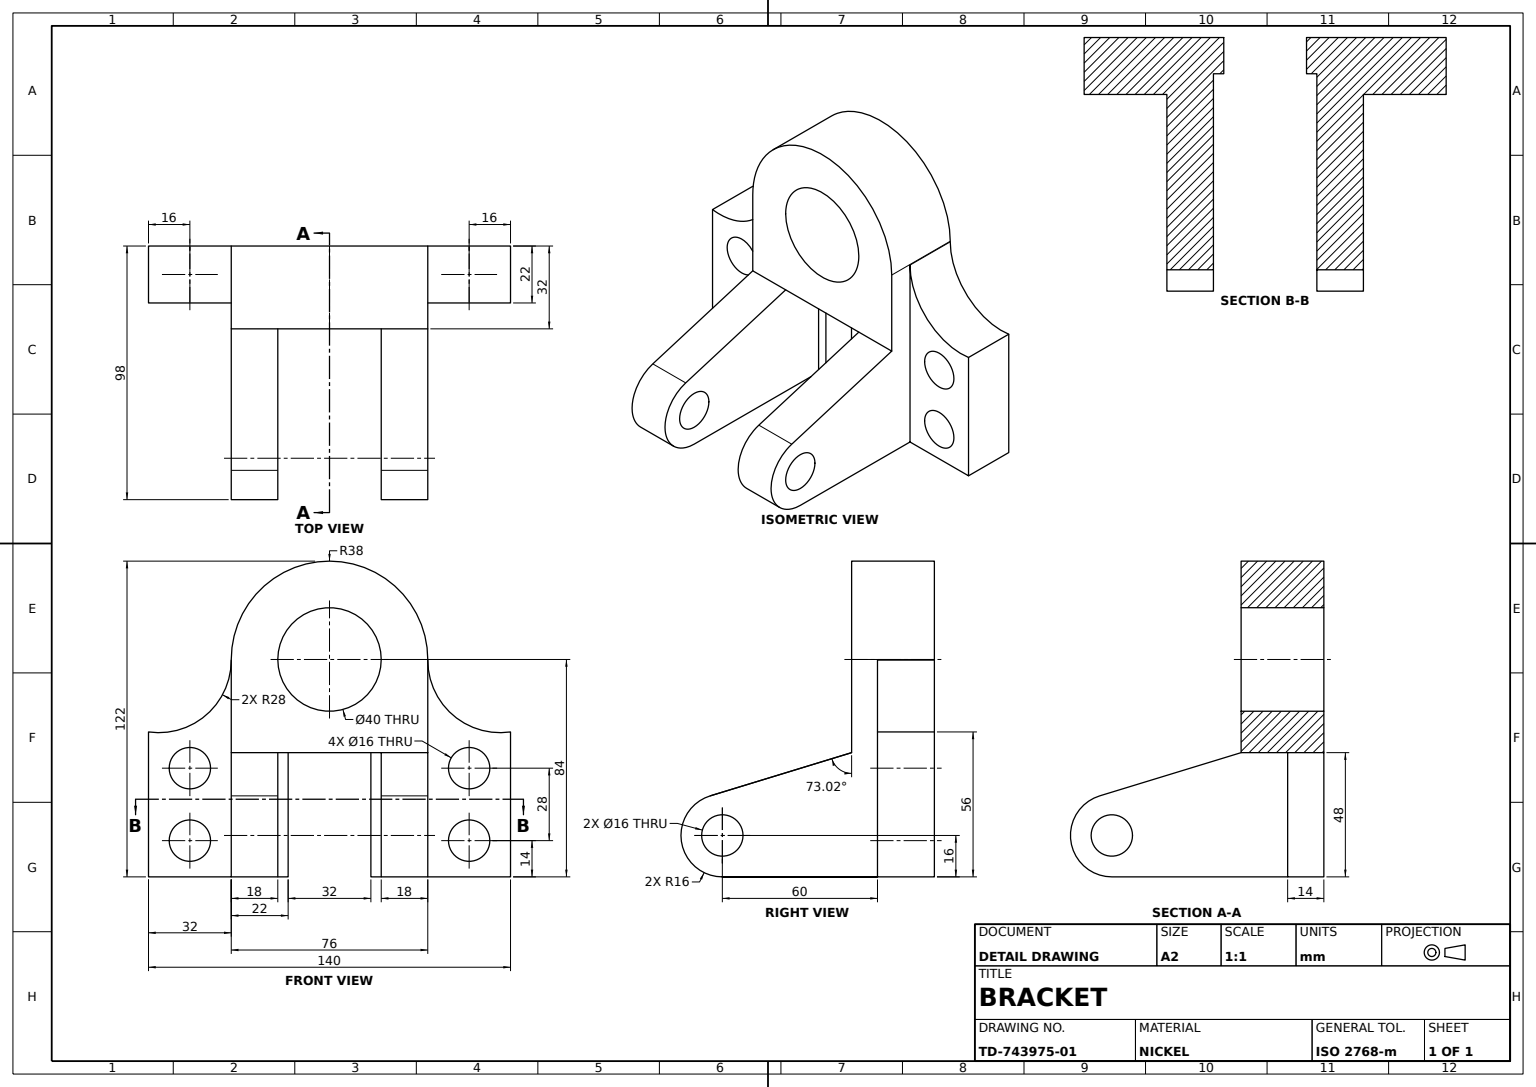
from build123d import *

# Parameters (mm, degrees)
BASE_BLOCK_SKETCH_R  = 20
BASE_BLOCK_DEPTH     = 32
PIVOT_BOSS_SKETCH_R  = 8
PIVOT_BOSS_DEPTH     = 22
ARM_START            = 20
ARM_PROFILE_SKETCH_R = 8
ARM_1_DEPTH          = 18
ARM_START_2          = -38
SKETCH3_2_R          = 8
ARM_2_DEPTH          = 18
SIDE_LUG_SKETCH_W    = 4
SIDE_LUG_SKETCH_H    = 48
SIDE_LUGS_DEPTH      = 14


with BuildPart() as part:
    # Base Block Sketch → Base Block (new body)
    with BuildSketch(Plane(origin=(0, 0, 0), x_dir=(0, 0, -1), z_dir=(1, 0, 0))):
        with BuildLine():
            Line((-38, 0), (-38, -36))
            Line((-38, -36), (38, -36))
            Line((38, -36), (38, 0))
            ThreePointArc((38, 0), (0, 38), (-38, 0))
        make_face()
        Circle(BASE_BLOCK_SKETCH_R, mode=Mode.SUBTRACT)
    extrude(amount=BASE_BLOCK_DEPTH)

    # Pivot Boss Sketch → Pivot Boss (add)
    # profile 1 of 2: a face of its own
    with BuildSketch(Plane(origin=(0, 0, 0), x_dir=(0, 0, -1), z_dir=(1, 0, 0))):
        with BuildLine():
            Line((-38, -0.287187079), (-38, -84))
            Line((-38, -84), (-70, -84))
            Line((-70, -84), (-70, -28))
            ThreePointArc((-70, -28), (-47.66969722, -21.453197567), (-38, -0.287187079))
        make_face()
        with Locations((-54, -42)):
            Circle(PIVOT_BOSS_SKETCH_R, mode=Mode.SUBTRACT)
        with Locations((-54, -70)):
            Circle(PIVOT_BOSS_SKETCH_R, mode=Mode.SUBTRACT)
    # profile 2 of 2: a face of its own
    with BuildSketch(Plane(origin=(0, 0, 0), x_dir=(0, 0, -1), z_dir=(1, 0, 0))):
        with BuildLine():
            Line((70, -28), (70, -84))
            Line((70, -84), (38, -84))
            Line((38, -84), (38, -0.287187079))
            ThreePointArc((38, -0.287187079), (47.66969722, -21.453197567), (70, -28))
        make_face()
        with Locations(Location((54, -70, 0), (0, 0, 180))):
            Circle(PIVOT_BOSS_SKETCH_R, mode=Mode.SUBTRACT)
        with Locations(Location((54, -42, 0), (0, 0, 180))):
            Circle(PIVOT_BOSS_SKETCH_R, mode=Mode.SUBTRACT)
    extrude(amount=PIVOT_BOSS_DEPTH)

    # Arm Profile Sketch → Arm 1 (add)
    with BuildSketch(Plane.XY.offset(ARM_START)):
        with BuildLine():
            Line((0, -84), (82, -84))
            ThreePointArc((82, -84), (97.824601816, -70.362620868), (86.673441811, -52.697747171))
            Line((86.673441811, -52.697747171), (32, -36))
            Line((32, -36), (0, -36))
            Line((0, -36), (0, -84))
        make_face()
        with Locations((82, -68)):
            Circle(ARM_PROFILE_SKETCH_R, mode=Mode.SUBTRACT)
    extrude(amount=ARM_1_DEPTH)

    # Sketch3_2 → Arm 2 (add)
    with BuildSketch(Plane.XY.offset(ARM_START_2)):
        with BuildLine():
            Line((0, -84), (82, -84))
            ThreePointArc((82, -84), (97.824601816, -70.362620868), (86.673441811, -52.697747171))
            Line((86.673441811, -52.697747171), (32, -36))
            Line((32, -36), (0, -36))
            Line((0, -36), (0, -84))
        make_face()
        with Locations((82, -68)):
            Circle(SKETCH3_2_R, mode=Mode.SUBTRACT)
    extrude(amount=ARM_2_DEPTH)

    # Side Lug Sketch → Side Lugs (add)
    with BuildSketch(Plane.ZY):
        with Locations((-18, -60)):
            Rectangle(SIDE_LUG_SKETCH_W, SIDE_LUG_SKETCH_H)
        with Locations((18, -60)):
            Rectangle(SIDE_LUG_SKETCH_W, SIDE_LUG_SKETCH_H)
    extrude(amount=-SIDE_LUGS_DEPTH)


solid = part.part
